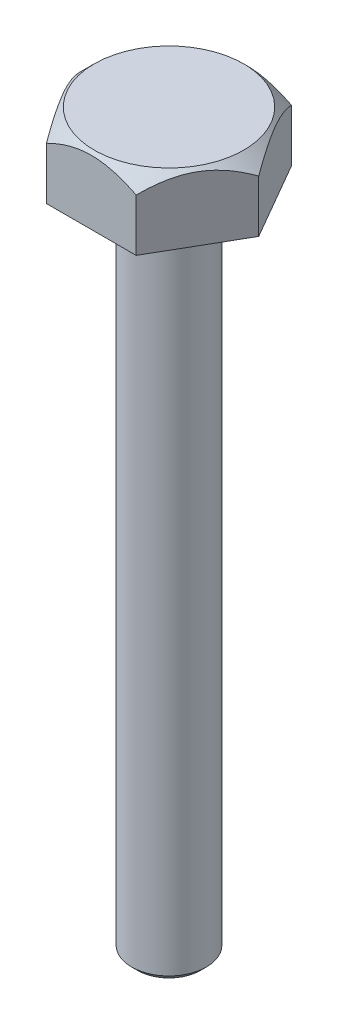
from build123d import *

# Parameters (mm, degrees)
HEX_HEAD_DEPTH              = 45
SHANK_SKETCH_50_R           = 25
SHANK_50X490_DEPTH          = 490
SHANK_END_CHAMFER_4X45_SIZE = 4


with BuildPart() as part:
    # Hex Head Sketch AF104 → Hex Head (new body)
    with BuildSketch(Plane(origin=(0, 0, 0), x_dir=(1, 0, 0), z_dir=(0, 1, 0))):
        Polygon((60.044427996, 0), (30.022213998, 52), (-30.022213998, 52), (-60.044427996, 0), (-30.022213998, -52), (30.022213998, -52), align=None)
    extrude(amount=-HEX_HEAD_DEPTH)

    # Head Chamfer Profile → Head Corner Chamfer Cut (revolve, cut)
    with BuildSketch(Plane.XY, mode=Mode.PRIVATE) as head_corner_chamfer_cut_sk:
        Polygon((50.044427996, 0), (60.044427996, 0), (60.044427996, -10), align=None)
    revolve(head_corner_chamfer_cut_sk.sketch.rotate(Axis((0, 0, 0), (0, -1, 0)), 180.000000001), axis=Axis((0, 0, 0), (0, -1, 0)), mode=Mode.SUBTRACT)

    # Shank Sketch Ø50 → Shank Ø50x490 (add)
    with BuildSketch(Plane(origin=(0, 0, 0), x_dir=(1, 0, 0), z_dir=(0, 1, 0))):
        with Locations(Location((0, 0, 0), (0, 0, 270))):
            Circle(SHANK_SKETCH_50_R)
    extrude(amount=-SHANK_50X490_DEPTH)

    # Shank End Chamfer 4x45°
    shank_end_chamfer_4x45_edges = [part.edges().sort_by_distance(p)[0] for p in [
        (0, -490, -25),
    ]]
    chamfer(shank_end_chamfer_4x45_edges, length=SHANK_END_CHAMFER_4X45_SIZE)


solid = part.part
